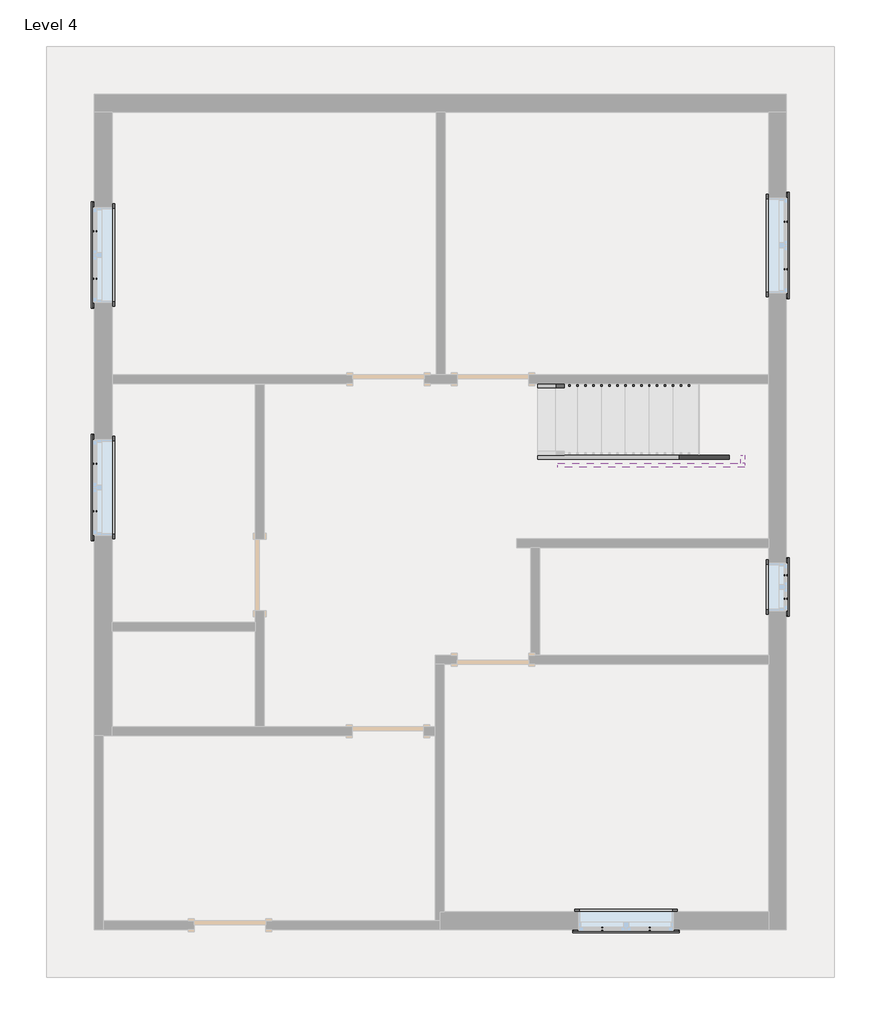
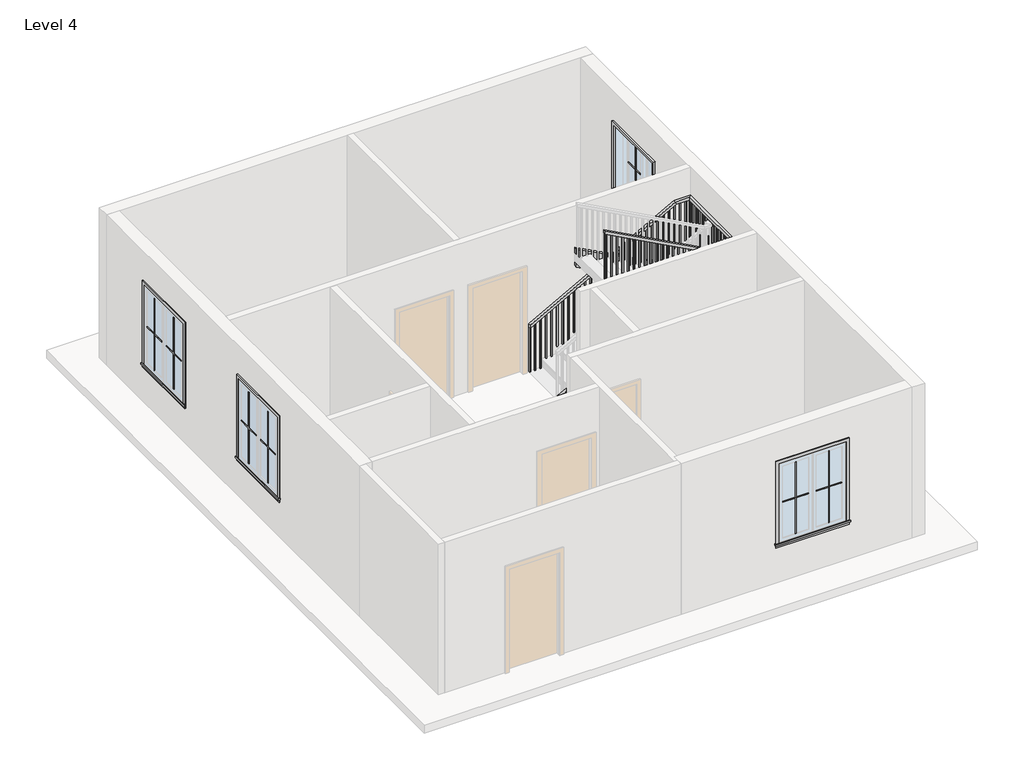
# One storey, part 2 of 2: 20 proxies, 3 members, 1 railing.
"""IFC4 building model written with IfcOpenShell, lengths in millimetres."""

from ifc_helpers import new_model, si_unit, frame, origin, place, context, project, spatial, polyline, outline, extrude, faceted_brep, transform, mapped, element, save
from components import muntin_pattern_2x2_muntin_pattern_2x2_6dad3731, muntin_pattern_2x2_muntin_pattern_2x2_a30a3345, muntin_pattern_2x2_muntin_pattern_2x2_53152e2c, muntin_pattern_2x2_muntin_pattern_2x2_e8f3e573, trim_window_exterior_flat_with_sill_92b9b949, trim_window_exterior_flat_with_sill_a665a915, trim_window_interior_flat_picture_frame_3bb882cf, trim_window_interior_flat_picture_frame_d485c387

model = new_model("IFC4")

# Units and contexts
model_context = context("Model", 3, world=origin())
ifc_project = project(units=[si_unit("LENGTHUNIT", "METRE", prefix="MILLI")], contexts=[model_context])

# Site, building, storey
site = spatial("IfcSite", under=ifc_project)
building = spatial("IfcBuilding", under=site)
storey = spatial("IfcBuildingStorey", under=building, Name="Level 4", Elevation=9144.0)

# Proxies
placement = place(None, origin())
muntin_pattern_2x2_muntin_pattern_2x2_shape = muntin_pattern_2x2_muntin_pattern_2x2_6dad3731(model_context)
element("IfcBuildingElementProxy", 1, Name="Muntin Pattern_2x2 : Muntin Pattern_2x2", ObjectType="Muntin Pattern_2x2 : Muntin Pattern_2x2", at=placement, inside=storey, context=model_context, shape_type="MappedRepresentation", body=[
    mapped(muntin_pattern_2x2_muntin_pattern_2x2_shape, transform((10003.63125, 2232.025, 10128.25), x_axis=(-1.0, 0.0, 0.0), y_axis=(0.0, -1.0, 0.0), z_axis=(0.0, 0.0, 1.0))),
])
element("IfcBuildingElementProxy", 2, Name="Muntin Pattern_2x2 : Muntin Pattern_2x2", ObjectType="Muntin Pattern_2x2 : Muntin Pattern_2x2", at=placement, inside=storey, context=model_context, shape_type="MappedRepresentation", body=[
    mapped(muntin_pattern_2x2_muntin_pattern_2x2_shape, transform((2917.825, 7567.6125, 10128.25), x_axis=(0.0, 1.0, 0.0), y_axis=(-1.0, 0.0, 0.0), z_axis=(0.0, 0.0, 1.0))),
])
element("IfcBuildingElementProxy", 3, Name="Muntin Pattern_2x2 : Muntin Pattern_2x2", ObjectType="Muntin Pattern_2x2 : Muntin Pattern_2x2", at=placement, inside=storey, context=model_context, shape_type="MappedRepresentation", body=[
    mapped(muntin_pattern_2x2_muntin_pattern_2x2_shape, transform((2917.825, 10536.2375, 10128.25), x_axis=(0.0, 1.0, 0.0), y_axis=(-1.0, 0.0, 0.0), z_axis=(0.0, 0.0, 1.0))),
])
element("IfcBuildingElementProxy", 4, Name="Muntin Pattern_2x2 : Muntin Pattern_2x2", ObjectType="Muntin Pattern_2x2 : Muntin Pattern_2x2", at=placement, inside=storey, context=model_context, shape_type="MappedRepresentation", body=[
    mapped(muntin_pattern_2x2_muntin_pattern_2x2_shape, transform((11737.975, 11264.9, 10128.25), x_axis=(0.0, -1.0, 0.0), y_axis=(1.0, 0.0, 0.0), z_axis=(0.0, 0.0, 1.0))),
])
muntin_pattern_2x2_muntin_pattern_2x2_2_shape = muntin_pattern_2x2_muntin_pattern_2x2_a30a3345(model_context)
element("IfcBuildingElementProxy", 5, Name="Muntin Pattern_2x2 : Muntin Pattern_2x2", ObjectType="Muntin Pattern_2x2 : Muntin Pattern_2x2", at=placement, inside=storey, context=model_context, shape_type="MappedRepresentation", body=[
    mapped(muntin_pattern_2x2_muntin_pattern_2x2_2_shape, transform((9397.20625, 2232.025, 10128.25), x_axis=(1.0, 0.0, 0.0), y_axis=(0.0, 1.0, 0.0), z_axis=(0.0, 0.0, 1.0))),
])
element("IfcBuildingElementProxy", 6, Name="Muntin Pattern_2x2 : Muntin Pattern_2x2", ObjectType="Muntin Pattern_2x2 : Muntin Pattern_2x2", at=placement, inside=storey, context=model_context, shape_type="MappedRepresentation", body=[
    mapped(muntin_pattern_2x2_muntin_pattern_2x2_2_shape, transform((2917.825, 8174.0375, 10128.25), x_axis=(0.0, -1.0, 0.0), y_axis=(1.0, 0.0, 0.0), z_axis=(0.0, 0.0, 1.0))),
])
element("IfcBuildingElementProxy", 7, Name="Muntin Pattern_2x2 : Muntin Pattern_2x2", ObjectType="Muntin Pattern_2x2 : Muntin Pattern_2x2", at=placement, inside=storey, context=model_context, shape_type="MappedRepresentation", body=[
    mapped(muntin_pattern_2x2_muntin_pattern_2x2_2_shape, transform((2917.825, 11142.6625, 10128.25), x_axis=(0.0, -1.0, 0.0), y_axis=(1.0, 0.0, 0.0), z_axis=(0.0, 0.0, 1.0))),
])
element("IfcBuildingElementProxy", 8, Name="Muntin Pattern_2x2 : Muntin Pattern_2x2", ObjectType="Muntin Pattern_2x2 : Muntin Pattern_2x2", at=placement, inside=storey, context=model_context, shape_type="MappedRepresentation", body=[
    mapped(muntin_pattern_2x2_muntin_pattern_2x2_2_shape, transform((11737.975, 10658.475, 10128.25), x_axis=(0.0, 1.0, 0.0), y_axis=(-1.0, 0.0, 0.0), z_axis=(0.0, 0.0, 1.0))),
])
muntin_pattern_2x2_muntin_pattern_2x2_3_shape = muntin_pattern_2x2_muntin_pattern_2x2_53152e2c(model_context)
element("IfcBuildingElementProxy", 9, Name="Muntin Pattern_2x2 : Muntin Pattern_2x2", ObjectType="Muntin Pattern_2x2 : Muntin Pattern_2x2", at=placement, inside=storey, context=model_context, shape_type="MappedRepresentation", body=[
    mapped(muntin_pattern_2x2_muntin_pattern_2x2_3_shape, transform((11737.975, 6748.4625, 10128.25), x_axis=(0.0, -1.0, 0.0), y_axis=(1.0, 0.0, 0.0), z_axis=(0.0, 0.0, 1.0))),
])
muntin_pattern_2x2_muntin_pattern_2x2_4_shape = muntin_pattern_2x2_muntin_pattern_2x2_e8f3e573(model_context)
element("IfcBuildingElementProxy", 10, Name="Muntin Pattern_2x2 : Muntin Pattern_2x2", ObjectType="Muntin Pattern_2x2 : Muntin Pattern_2x2", at=placement, inside=storey, context=model_context, shape_type="MappedRepresentation", body=[
    mapped(muntin_pattern_2x2_muntin_pattern_2x2_4_shape, transform((11737.975, 6446.8375, 10128.25), x_axis=(0.0, 1.0, 0.0), y_axis=(-1.0, 0.0, 0.0), z_axis=(0.0, 0.0, 1.0))),
])
trim_window_exterior_flat_with_sill_shape = trim_window_exterior_flat_with_sill_92b9b949(model_context)
element("IfcBuildingElementProxy", 11, Name="Trim-Window-Exterior-Flat : with Sill", ObjectType="Trim-Window-Exterior-Flat : with Sill", at=placement, inside=storey, context=model_context, shape_type="MappedRepresentation", body=[
    mapped(trim_window_exterior_flat_with_sill_shape, transform((9700.41875, 2222.5, 11582.4), x_axis=(1.0, 0.0, 0.0), y_axis=(0.0, 0.0, 1.0), z_axis=(0.0, -1.0, 0.0))),
])
element("IfcBuildingElementProxy", 12, Name="Trim-Window-Exterior-Flat : with Sill", ObjectType="Trim-Window-Exterior-Flat : with Sill", at=placement, inside=storey, context=model_context, shape_type="MappedRepresentation", body=[
    mapped(trim_window_exterior_flat_with_sill_shape, transform((2908.3, 7870.825, 11582.4), x_axis=(0.0, -1.0, 0.0), y_axis=(0.0, 0.0, 1.0), z_axis=(-1.0, 0.0, 0.0))),
])
element("IfcBuildingElementProxy", 13, Name="Trim-Window-Exterior-Flat : with Sill", ObjectType="Trim-Window-Exterior-Flat : with Sill", at=placement, inside=storey, context=model_context, shape_type="MappedRepresentation", body=[
    mapped(trim_window_exterior_flat_with_sill_shape, transform((2908.3, 10839.45, 11582.4), x_axis=(0.0, -1.0, 0.0), y_axis=(0.0, 0.0, 1.0), z_axis=(-1.0, 0.0, 0.0))),
])
element("IfcBuildingElementProxy", 14, Name="Trim-Window-Exterior-Flat : with Sill", ObjectType="Trim-Window-Exterior-Flat : with Sill", at=placement, inside=storey, context=model_context, shape_type="MappedRepresentation", body=[
    mapped(trim_window_exterior_flat_with_sill_shape, transform((11747.5, 10961.6875, 11582.4), x_axis=(0.0, 1.0, 0.0), y_axis=(0.0, 0.0, 1.0), z_axis=(1.0, 0.0, 0.0))),
])
trim_window_exterior_flat_with_sill_2_shape = trim_window_exterior_flat_with_sill_a665a915(model_context)
element("IfcBuildingElementProxy", 15, Name="Trim-Window-Exterior-Flat : with Sill", ObjectType="Trim-Window-Exterior-Flat : with Sill", at=placement, inside=storey, context=model_context, shape_type="MappedRepresentation", body=[
    mapped(trim_window_exterior_flat_with_sill_2_shape, transform((11747.5, 6597.65, 10972.8), x_axis=(0.0, 1.0, 0.0), y_axis=(0.0, 0.0, 1.0), z_axis=(1.0, 0.0, 0.0))),
])
trim_window_interior_flat_picture_frame_shape = trim_window_interior_flat_picture_frame_3bb882cf(model_context)
element("IfcBuildingElementProxy", 16, Name="Trim-Window-Interior-Flat : Picture Frame", ObjectType="Trim-Window-Interior-Flat : Picture Frame", at=placement, inside=storey, context=model_context, shape_type="MappedRepresentation", body=[
    mapped(trim_window_interior_flat_picture_frame_shape, transform((9700.41875, 2451.1, 11582.4), x_axis=(-1.0, 0.0, 0.0), y_axis=(0.0, 0.0, 1.0), z_axis=(0.0, 1.0, 0.0))),
])
element("IfcBuildingElementProxy", 17, Name="Trim-Window-Interior-Flat : Picture Frame", ObjectType="Trim-Window-Interior-Flat : Picture Frame", at=placement, inside=storey, context=model_context, shape_type="MappedRepresentation", body=[
    mapped(trim_window_interior_flat_picture_frame_shape, transform((3136.9, 7870.825, 11582.4), x_axis=(0.0, 1.0, 0.0), y_axis=(0.0, 0.0, 1.0), z_axis=(1.0, 0.0, 0.0))),
])
element("IfcBuildingElementProxy", 18, Name="Trim-Window-Interior-Flat : Picture Frame", ObjectType="Trim-Window-Interior-Flat : Picture Frame", at=placement, inside=storey, context=model_context, shape_type="MappedRepresentation", body=[
    mapped(trim_window_interior_flat_picture_frame_shape, transform((3136.9, 10839.45, 11582.4), x_axis=(0.0, 1.0, 0.0), y_axis=(0.0, 0.0, 1.0), z_axis=(1.0, 0.0, 0.0))),
])
element("IfcBuildingElementProxy", 19, Name="Trim-Window-Interior-Flat : Picture Frame", ObjectType="Trim-Window-Interior-Flat : Picture Frame", at=placement, inside=storey, context=model_context, shape_type="MappedRepresentation", body=[
    mapped(trim_window_interior_flat_picture_frame_shape, transform((11518.9, 10961.6875, 11582.4), x_axis=(0.0, -1.0, 0.0), y_axis=(0.0, 0.0, 1.0), z_axis=(-1.0, 0.0, 0.0))),
])
trim_window_interior_flat_picture_frame_2_shape = trim_window_interior_flat_picture_frame_d485c387(model_context)
element("IfcBuildingElementProxy", 20, Name="Trim-Window-Interior-Flat : Picture Frame", ObjectType="Trim-Window-Interior-Flat : Picture Frame", at=placement, inside=storey, context=model_context, shape_type="MappedRepresentation", body=[
    mapped(trim_window_interior_flat_picture_frame_2_shape, transform((11518.9, 6597.65, 10972.8), x_axis=(0.0, -1.0, 0.0), y_axis=(0.0, 0.0, 1.0), z_axis=(-1.0, 0.0, 0.0))),
])

# Members
element("IfcMember", 21, ObjectType="Stringer - 2\" Width", at=placement, inside=storey, context=model_context, shape_type="SweptSolid", body=[
    extrude(outline(polyline([(9388.4581083, 8572.5), (9144.0, 8572.5), (9144.0, 8761.9689927), (10421.1621978, 11163.3), (10766.3905183, 11163.3), (9388.4581083, 8572.5)])), frame((0.0, 8229.6, 0.0), z_axis=(0.0, 1.0, 0.0), x_axis=(0.0, 0.0, 1.0)), (0.0, 0.0, 1.0), 50.8),
])
element("IfcMember", 22, ObjectType="Stringer - 2\" Width", at=placement, inside=storey, context=model_context, shape_type="SweptSolid", body=[
    extrude(outline(polyline([(11163.3, 8280.4), (11214.1, 8280.4), (11214.1, 8178.8), (11163.3, 8178.8), (11163.3, 8280.4)])), frame((0.0, 0.0, 10519.6105263), z_axis=(0.0, 0.0, 1.0), x_axis=(1.0, 0.0, 0.0)), (0.0, 0.0, 1.0), 304.8),
])
element("IfcMember", 23, ObjectType="Stringer - 2\" Width", at=placement, inside=storey, context=model_context, shape_type="SweptSolid", body=[
    extrude(outline(polyline([(10608.9419568, 11214.1), (10953.380564, 11214.1), (12210.012143, 8826.5), (11865.5735358, 8826.5), (10608.9419568, 11214.1)])), frame((0.0, 8128.0, 0.0), z_axis=(0.0, 1.0, 0.0), x_axis=(0.0, 0.0, 1.0)), (0.0, 0.0, 1.0), 50.8),
])

# Railing
element("IfcRailing", 24, ObjectType="Handrail - Rectangular", at=placement, inside=storey, context=model_context, shape_type="SolidModel", body=[
    faceted_brep([(8572.5, 9194.8, 10218.8210526), (8572.5, 9194.8, 10160.9285199), (8572.5, 9144.0, 10160.9285199), (8572.5, 9144.0, 10218.8210526), (11214.1, 9194.8, 11662.6105263), (11227.076708, 9194.8, 11611.8105263), (11227.076708, 9144.0, 11611.8105263), (11214.1, 9144.0, 11662.6105263), (11518.9, 9194.8, 11662.6105263), (11518.9, 9194.8, 11611.8105263), (11468.1, 9144.0, 11611.8105263), (11468.1, 9144.0, 11662.6105263), (11518.9, 7340.6, 11662.6105263), (11518.9, 7289.8, 11611.8105263), (11468.1, 7289.8, 11611.8105263), (11468.1, 7340.6, 11662.6105263), (11518.9, 7340.6, 11727.4615901), (11518.9, 7289.8, 11676.6615901), (11468.1, 7289.8, 11676.6615901), (11468.1, 7340.6, 11727.4615901), (11518.9, 7213.6, 11727.4615901), (11518.9, 7213.6, 11676.6615901), (11468.1, 7264.4, 11676.6615901), (11468.1, 7264.4, 11727.4615901), (11391.9, 7213.6, 11727.4615901), (11379.1122768, 7213.6, 11676.6615901), (11379.1122768, 7264.4, 11676.6615901), (11391.9, 7264.4, 11727.4615901), (8826.5, 7213.6, 13106.4), (8826.5, 7264.4, 13106.4), (8826.5, 7264.4, 13048.7264198), (8826.5, 7213.6, 13048.7264198)], [[[0, 1, 2, 3]], [[1, 0, 4, 5]], [[2, 1, 5, 6]], [[3, 2, 6, 7]], [[0, 3, 7, 4]], [[5, 4, 8, 9]], [[6, 5, 9, 10]], [[7, 6, 10, 11]], [[4, 7, 11, 8]], [[9, 8, 12, 13]], [[10, 9, 13, 14]], [[11, 10, 14, 15]], [[8, 11, 15, 12]], [[13, 12, 16, 17]], [[14, 13, 17, 18]], [[15, 14, 18, 19]], [[12, 15, 19, 16]], [[17, 16, 20, 21]], [[18, 17, 21, 22]], [[19, 18, 22, 23]], [[16, 19, 23, 20]], [[21, 20, 24, 25]], [[22, 21, 25, 26]], [[23, 22, 26, 27]], [[20, 23, 27, 24]], [[28, 29, 30, 31]], [[25, 24, 28, 31]], [[26, 25, 31, 30]], [[27, 26, 30, 29]], [[24, 27, 29, 28]]]),
    extrude(outline(polyline([(13040.193385, 8842.375), (12031.5789474, 8842.375), (12031.5789474, 8861.425), (13029.9537434, 8861.425), (13040.193385, 8842.375)])), frame((0.0, 7229.475, 0.0), z_axis=(0.0, 1.0, 0.0), x_axis=(0.0, 0.0, 1.0)), (0.0, 0.0, 1.0), 19.05),
    extrude(outline(polyline([(12985.5819629, 8943.975), (12031.5789474, 8943.975), (12031.5789474, 8963.025), (12975.3423212, 8963.025), (12985.5819629, 8943.975)])), frame((0.0, 7229.475, 0.0), z_axis=(0.0, 1.0, 0.0), x_axis=(0.0, 0.0, 1.0)), (0.0, 0.0, 1.0), 19.05),
    extrude(outline(polyline([(12930.9705407, 9045.575), (12031.5789474, 9045.575), (12031.5789474, 9064.625), (12920.730899, 9064.625), (12930.9705407, 9045.575)])), frame((0.0, 7229.475, 0.0), z_axis=(0.0, 1.0, 0.0), x_axis=(0.0, 0.0, 1.0)), (0.0, 0.0, 1.0), 19.05),
    extrude(outline(polyline([(12876.3591185, 9147.175), (11871.1578947, 9147.175), (11871.1578947, 9166.225), (12866.1194769, 9166.225), (12876.3591185, 9147.175)])), frame((0.0, 7229.475, 0.0), z_axis=(0.0, 1.0, 0.0), x_axis=(0.0, 0.0, 1.0)), (0.0, 0.0, 1.0), 19.05),
    extrude(outline(polyline([(12821.7476964, 9248.775), (11871.1578947, 9248.775), (11871.1578947, 9267.825), (12811.5080547, 9267.825), (12821.7476964, 9248.775)])), frame((0.0, 7229.475, 0.0), z_axis=(0.0, 1.0, 0.0), x_axis=(0.0, 0.0, 1.0)), (0.0, 0.0, 1.0), 19.05),
    extrude(outline(polyline([(12767.1362742, 9350.375), (11871.1578947, 9350.375), (11871.1578947, 9369.425), (12756.8966325, 9369.425), (12767.1362742, 9350.375)])), frame((0.0, 7229.475, 0.0), z_axis=(0.0, 1.0, 0.0), x_axis=(0.0, 0.0, 1.0)), (0.0, 0.0, 1.0), 19.05),
    extrude(outline(polyline([(12712.524852, 9451.975), (11710.7368421, 9451.975), (11710.7368421, 9471.025), (12702.2852104, 9471.025), (12712.524852, 9451.975)])), frame((0.0, 7229.475, 0.0), z_axis=(0.0, 1.0, 0.0), x_axis=(0.0, 0.0, 1.0)), (0.0, 0.0, 1.0), 19.05),
    extrude(outline(polyline([(12657.9134298, 9553.575), (11710.7368421, 9553.575), (11710.7368421, 9572.625), (12647.6737882, 9572.625), (12657.9134298, 9553.575)])), frame((0.0, 7229.475, 0.0), z_axis=(0.0, 1.0, 0.0), x_axis=(0.0, 0.0, 1.0)), (0.0, 0.0, 1.0), 19.05),
    extrude(outline(polyline([(12603.3004835, 9655.175), (11710.7368421, 9655.175), (11710.7368421, 9674.225), (12592.8885402, 9674.225), (12603.3004835, 9655.175)])), frame((0.0, 7229.475, 0.0), z_axis=(0.0, 1.0, 0.0), x_axis=(0.0, 0.0, 1.0)), (0.0, 0.0, 1.0), 19.05),
    extrude(outline(polyline([(12548.6905855, 9756.775), (11550.3157895, 9756.775), (11550.3157895, 9775.825), (12538.4509438, 9775.825), (12548.6905855, 9756.775)])), frame((0.0, 7229.475, 0.0), z_axis=(0.0, 1.0, 0.0), x_axis=(0.0, 0.0, 1.0)), (0.0, 0.0, 1.0), 19.05),
    extrude(outline(polyline([(12494.0791633, 9858.375), (11550.3157895, 9858.375), (11550.3157895, 9877.425), (12483.8395217, 9877.425), (12494.0791633, 9858.375)])), frame((0.0, 7229.475, 0.0), z_axis=(0.0, 1.0, 0.0), x_axis=(0.0, 0.0, 1.0)), (0.0, 0.0, 1.0), 19.05),
    extrude(outline(polyline([(12439.4677411, 9959.975), (11550.3157895, 9959.975), (11550.3157895, 9979.025), (12429.2280995, 9979.025), (12439.4677411, 9959.975)])), frame((0.0, 7229.475, 0.0), z_axis=(0.0, 1.0, 0.0), x_axis=(0.0, 0.0, 1.0)), (0.0, 0.0, 1.0), 19.05),
    extrude(outline(polyline([(12384.856319, 10061.575), (11389.8947368, 10061.575), (11389.8947368, 10080.625), (12374.6166773, 10080.625), (12384.856319, 10061.575)])), frame((0.0, 7229.475, 0.0), z_axis=(0.0, 1.0, 0.0), x_axis=(0.0, 0.0, 1.0)), (0.0, 0.0, 1.0), 19.05),
    extrude(outline(polyline([(12330.2448968, 10163.175), (11389.8947368, 10163.175), (11389.8947368, 10182.225), (12320.0052551, 10182.225), (12330.2448968, 10163.175)])), frame((0.0, 7229.475, 0.0), z_axis=(0.0, 1.0, 0.0), x_axis=(0.0, 0.0, 1.0)), (0.0, 0.0, 1.0), 19.05),
    extrude(outline(polyline([(12275.6334746, 10264.775), (11389.8947368, 10264.775), (11389.8947368, 10283.825), (12265.393833, 10283.825), (12275.6334746, 10264.775)])), frame((0.0, 7229.475, 0.0), z_axis=(0.0, 1.0, 0.0), x_axis=(0.0, 0.0, 1.0)), (0.0, 0.0, 1.0), 19.05),
    extrude(outline(polyline([(12221.0220525, 10366.375), (11229.4736842, 10366.375), (11229.4736842, 10385.425), (12210.7824108, 10385.425), (12221.0220525, 10366.375)])), frame((0.0, 7229.475, 0.0), z_axis=(0.0, 1.0, 0.0), x_axis=(0.0, 0.0, 1.0)), (0.0, 0.0, 1.0), 19.05),
    extrude(outline(polyline([(12166.4106303, 10467.975), (11229.4736842, 10467.975), (11229.4736842, 10487.025), (12156.1709886, 10487.025), (12166.4106303, 10467.975)])), frame((0.0, 7229.475, 0.0), z_axis=(0.0, 1.0, 0.0), x_axis=(0.0, 0.0, 1.0)), (0.0, 0.0, 1.0), 19.05),
    extrude(outline(polyline([(12111.7992081, 10569.575), (11229.4736842, 10569.575), (11229.4736842, 10588.625), (12101.5595665, 10588.625), (12111.7992081, 10569.575)])), frame((0.0, 7229.475, 0.0), z_axis=(0.0, 1.0, 0.0), x_axis=(0.0, 0.0, 1.0)), (0.0, 0.0, 1.0), 19.05),
    extrude(outline(polyline([(12057.1877859, 10671.175), (11069.0526316, 10671.175), (11069.0526316, 10690.225), (12046.9481443, 10690.225), (12057.1877859, 10671.175)])), frame((0.0, 7229.475, 0.0), z_axis=(0.0, 1.0, 0.0), x_axis=(0.0, 0.0, 1.0)), (0.0, 0.0, 1.0), 19.05),
    extrude(outline(polyline([(12002.5763638, 10772.775), (11069.0526316, 10772.775), (11069.0526316, 10791.825), (11992.3367221, 10791.825), (12002.5763638, 10772.775)])), frame((0.0, 7229.475, 0.0), z_axis=(0.0, 1.0, 0.0), x_axis=(0.0, 0.0, 1.0)), (0.0, 0.0, 1.0), 19.05),
    extrude(outline(polyline([(11947.9649416, 10874.375), (11069.0526316, 10874.375), (11069.0526316, 10893.425), (11937.7252999, 10893.425), (11947.9649416, 10874.375)])), frame((0.0, 7229.475, 0.0), z_axis=(0.0, 1.0, 0.0), x_axis=(0.0, 0.0, 1.0)), (0.0, 0.0, 1.0), 19.05),
    extrude(outline(polyline([(11893.3535194, 10975.975), (10908.6315789, 10975.975), (10908.6315789, 10995.025), (11883.1138778, 10995.025), (11893.3535194, 10975.975)])), frame((0.0, 7229.475, 0.0), z_axis=(0.0, 1.0, 0.0), x_axis=(0.0, 0.0, 1.0)), (0.0, 0.0, 1.0), 19.05),
    extrude(outline(polyline([(11838.7420972, 11077.575), (10908.6315789, 11077.575), (10908.6315789, 11096.625), (11828.5024556, 11096.625), (11838.7420972, 11077.575)])), frame((0.0, 7229.475, 0.0), z_axis=(0.0, 1.0, 0.0), x_axis=(0.0, 0.0, 1.0)), (0.0, 0.0, 1.0), 19.05),
    extrude(outline(polyline([(11784.1306751, 11179.175), (10908.6315789, 11179.175), (10908.6315789, 11198.225), (11773.8910334, 11198.225), (11784.1306751, 11179.175)])), frame((0.0, 7229.475, 0.0), z_axis=(0.0, 1.0, 0.0), x_axis=(0.0, 0.0, 1.0)), (0.0, 0.0, 1.0), 19.05),
    extrude(outline(polyline([(11729.5192529, 11280.775), (10748.2105263, 11280.775), (10748.2105263, 11299.825), (11719.2796112, 11299.825), (11729.5192529, 11280.775)])), frame((0.0, 7229.475, 0.0), z_axis=(0.0, 1.0, 0.0), x_axis=(0.0, 0.0, 1.0)), (0.0, 0.0, 1.0), 19.05),
    extrude(outline(polyline([(11674.9078307, 11382.375), (10748.2105263, 11382.375), (10748.2105263, 11401.425), (11664.6681891, 11401.425), (11674.9078307, 11382.375)])), frame((0.0, 7229.475, 0.0), z_axis=(0.0, 1.0, 0.0), x_axis=(0.0, 0.0, 1.0)), (0.0, 0.0, 1.0), 19.05),
    extrude(outline(polyline([(11503.025, 7350.125), (11503.025, 7331.075), (11483.975, 7331.075), (11483.975, 7350.125), (11503.025, 7350.125)])), frame((0.0, 0.0, 10748.2105263), z_axis=(0.0, 0.0, 1.0), x_axis=(1.0, 0.0, 0.0)), (0.0, 0.0, 1.0), 863.6),
    extrude(outline(polyline([(11503.025, 7451.725), (11503.025, 7432.675), (11483.975, 7432.675), (11483.975, 7451.725), (11503.025, 7451.725)])), frame((0.0, 0.0, 10748.2105263), z_axis=(0.0, 0.0, 1.0), x_axis=(1.0, 0.0, 0.0)), (0.0, 0.0, 1.0), 863.6),
    extrude(outline(polyline([(11503.025, 7553.325), (11503.025, 7534.275), (11483.975, 7534.275), (11483.975, 7553.325), (11503.025, 7553.325)])), frame((0.0, 0.0, 10748.2105263), z_axis=(0.0, 0.0, 1.0), x_axis=(1.0, 0.0, 0.0)), (0.0, 0.0, 1.0), 863.6),
    extrude(outline(polyline([(11503.025, 7654.925), (11503.025, 7635.875), (11483.975, 7635.875), (11483.975, 7654.925), (11503.025, 7654.925)])), frame((0.0, 0.0, 10748.2105263), z_axis=(0.0, 0.0, 1.0), x_axis=(1.0, 0.0, 0.0)), (0.0, 0.0, 1.0), 863.6),
    extrude(outline(polyline([(11503.025, 7756.525), (11503.025, 7737.475), (11483.975, 7737.475), (11483.975, 7756.525), (11503.025, 7756.525)])), frame((0.0, 0.0, 10748.2105263), z_axis=(0.0, 0.0, 1.0), x_axis=(1.0, 0.0, 0.0)), (0.0, 0.0, 1.0), 863.6),
    extrude(outline(polyline([(11503.025, 7858.125), (11503.025, 7839.075), (11483.975, 7839.075), (11483.975, 7858.125), (11503.025, 7858.125)])), frame((0.0, 0.0, 10748.2105263), z_axis=(0.0, 0.0, 1.0), x_axis=(1.0, 0.0, 0.0)), (0.0, 0.0, 1.0), 863.6),
    extrude(outline(polyline([(11503.025, 7959.725), (11503.025, 7940.675), (11483.975, 7940.675), (11483.975, 7959.725), (11503.025, 7959.725)])), frame((0.0, 0.0, 10748.2105263), z_axis=(0.0, 0.0, 1.0), x_axis=(1.0, 0.0, 0.0)), (0.0, 0.0, 1.0), 863.6),
    extrude(outline(polyline([(11503.025, 8061.325), (11503.025, 8042.275), (11483.975, 8042.275), (11483.975, 8061.325), (11503.025, 8061.325)])), frame((0.0, 0.0, 10748.2105263), z_axis=(0.0, 0.0, 1.0), x_axis=(1.0, 0.0, 0.0)), (0.0, 0.0, 1.0), 863.6),
    extrude(outline(polyline([(11503.025, 8162.925), (11503.025, 8143.875), (11483.975, 8143.875), (11483.975, 8162.925), (11503.025, 8162.925)])), frame((0.0, 0.0, 10748.2105263), z_axis=(0.0, 0.0, 1.0), x_axis=(1.0, 0.0, 0.0)), (0.0, 0.0, 1.0), 863.6),
    extrude(outline(polyline([(11503.025, 8264.525), (11503.025, 8245.475), (11483.975, 8245.475), (11483.975, 8264.525), (11503.025, 8264.525)])), frame((0.0, 0.0, 10748.2105263), z_axis=(0.0, 0.0, 1.0), x_axis=(1.0, 0.0, 0.0)), (0.0, 0.0, 1.0), 863.6),
    extrude(outline(polyline([(11503.025, 8366.125), (11503.025, 8347.075), (11483.975, 8347.075), (11483.975, 8366.125), (11503.025, 8366.125)])), frame((0.0, 0.0, 10748.2105263), z_axis=(0.0, 0.0, 1.0), x_axis=(1.0, 0.0, 0.0)), (0.0, 0.0, 1.0), 863.6),
    extrude(outline(polyline([(11503.025, 8467.725), (11503.025, 8448.675), (11483.975, 8448.675), (11483.975, 8467.725), (11503.025, 8467.725)])), frame((0.0, 0.0, 10748.2105263), z_axis=(0.0, 0.0, 1.0), x_axis=(1.0, 0.0, 0.0)), (0.0, 0.0, 1.0), 863.6),
    extrude(outline(polyline([(11503.025, 8569.325), (11503.025, 8550.275), (11483.975, 8550.275), (11483.975, 8569.325), (11503.025, 8569.325)])), frame((0.0, 0.0, 10748.2105263), z_axis=(0.0, 0.0, 1.0), x_axis=(1.0, 0.0, 0.0)), (0.0, 0.0, 1.0), 863.6),
    extrude(outline(polyline([(11503.025, 8670.925), (11503.025, 8651.875), (11483.975, 8651.875), (11483.975, 8670.925), (11503.025, 8670.925)])), frame((0.0, 0.0, 10748.2105263), z_axis=(0.0, 0.0, 1.0), x_axis=(1.0, 0.0, 0.0)), (0.0, 0.0, 1.0), 863.6),
    extrude(outline(polyline([(11503.025, 8772.525), (11503.025, 8753.475), (11483.975, 8753.475), (11483.975, 8772.525), (11503.025, 8772.525)])), frame((0.0, 0.0, 10748.2105263), z_axis=(0.0, 0.0, 1.0), x_axis=(1.0, 0.0, 0.0)), (0.0, 0.0, 1.0), 863.6),
    extrude(outline(polyline([(11503.025, 8874.125), (11503.025, 8855.075), (11483.975, 8855.075), (11483.975, 8874.125), (11503.025, 8874.125)])), frame((0.0, 0.0, 10748.2105263), z_axis=(0.0, 0.0, 1.0), x_axis=(1.0, 0.0, 0.0)), (0.0, 0.0, 1.0), 863.6),
    extrude(outline(polyline([(11503.025, 8975.725), (11503.025, 8956.675), (11483.975, 8956.675), (11483.975, 8975.725), (11503.025, 8975.725)])), frame((0.0, 0.0, 10748.2105263), z_axis=(0.0, 0.0, 1.0), x_axis=(1.0, 0.0, 0.0)), (0.0, 0.0, 1.0), 863.6),
    extrude(outline(polyline([(11503.025, 9077.325), (11503.025, 9058.275), (11483.975, 9058.275), (11483.975, 9077.325), (11503.025, 9077.325)])), frame((0.0, 0.0, 10748.2105263), z_axis=(0.0, 0.0, 1.0), x_axis=(1.0, 0.0, 0.0)), (0.0, 0.0, 1.0), 863.6),
    extrude(outline(polyline([(11407.775, 9178.925), (11426.825, 9178.925), (11426.825, 9159.875), (11407.775, 9159.875), (11407.775, 9178.925)])), frame((0.0, 0.0, 10748.2105263), z_axis=(0.0, 0.0, 1.0), x_axis=(1.0, 0.0, 0.0)), (0.0, 0.0, 1.0), 863.6),
    extrude(outline(polyline([(11306.175, 9178.925), (11325.225, 9178.925), (11325.225, 9159.875), (11306.175, 9159.875), (11306.175, 9178.925)])), frame((0.0, 0.0, 10748.2105263), z_axis=(0.0, 0.0, 1.0), x_axis=(1.0, 0.0, 0.0)), (0.0, 0.0, 1.0), 863.6),
    extrude(outline(polyline([(11599.512022, 11204.575), (10748.2105263, 11204.575), (10748.2105263, 11223.625), (11609.9239653, 11223.625), (11599.512022, 11204.575)])), frame((0.0, 9159.875, 0.0), z_axis=(0.0, 1.0, 0.0), x_axis=(0.0, 0.0, 1.0)), (0.0, 0.0, 1.0), 19.05),
    extrude(outline(polyline([(11543.9816576, 11102.975), (10587.7894737, 11102.975), (10587.7894737, 11122.025), (11554.3936009, 11122.025), (11543.9816576, 11102.975)])), frame((0.0, 9159.875, 0.0), z_axis=(0.0, 1.0, 0.0), x_axis=(0.0, 0.0, 1.0)), (0.0, 0.0, 1.0), 19.05),
    extrude(outline(polyline([(11488.4512932, 11001.375), (10587.7894737, 11001.375), (10587.7894737, 11020.425), (11498.8632365, 11020.425), (11488.4512932, 11001.375)])), frame((0.0, 9159.875, 0.0), z_axis=(0.0, 1.0, 0.0), x_axis=(0.0, 0.0, 1.0)), (0.0, 0.0, 1.0), 19.05),
    extrude(outline(polyline([(11432.9209288, 10899.775), (10587.7894737, 10899.775), (10587.7894737, 10918.825), (11443.3328722, 10918.825), (11432.9209288, 10899.775)])), frame((0.0, 9159.875, 0.0), z_axis=(0.0, 1.0, 0.0), x_axis=(0.0, 0.0, 1.0)), (0.0, 0.0, 1.0), 19.05),
    extrude(outline(polyline([(11377.3905645, 10798.175), (10427.3684211, 10798.175), (10427.3684211, 10817.225), (11387.8025078, 10817.225), (11377.3905645, 10798.175)])), frame((0.0, 9159.875, 0.0), z_axis=(0.0, 1.0, 0.0), x_axis=(0.0, 0.0, 1.0)), (0.0, 0.0, 1.0), 19.05),
    extrude(outline(polyline([(11321.8602001, 10696.575), (10427.3684211, 10696.575), (10427.3684211, 10715.625), (11332.2721434, 10715.625), (11321.8602001, 10696.575)])), frame((0.0, 9159.875, 0.0), z_axis=(0.0, 1.0, 0.0), x_axis=(0.0, 0.0, 1.0)), (0.0, 0.0, 1.0), 19.05),
    extrude(outline(polyline([(11266.3298357, 10594.975), (10427.3684211, 10594.975), (10427.3684211, 10614.025), (11276.741779, 10614.025), (11266.3298357, 10594.975)])), frame((0.0, 9159.875, 0.0), z_axis=(0.0, 1.0, 0.0), x_axis=(0.0, 0.0, 1.0)), (0.0, 0.0, 1.0), 19.05),
    extrude(outline(polyline([(11210.7994714, 10493.375), (10266.9473684, 10493.375), (10266.9473684, 10512.425), (11221.2114147, 10512.425), (11210.7994714, 10493.375)])), frame((0.0, 9159.875, 0.0), z_axis=(0.0, 1.0, 0.0), x_axis=(0.0, 0.0, 1.0)), (0.0, 0.0, 1.0), 19.05),
    extrude(outline(polyline([(11155.269107, 10391.775), (10266.9473684, 10391.775), (10266.9473684, 10410.825), (11165.6810503, 10410.825), (11155.269107, 10391.775)])), frame((0.0, 9159.875, 0.0), z_axis=(0.0, 1.0, 0.0), x_axis=(0.0, 0.0, 1.0)), (0.0, 0.0, 1.0), 19.05),
    extrude(outline(polyline([(11099.7387426, 10290.175), (10266.9473684, 10290.175), (10266.9473684, 10309.225), (11110.1506859, 10309.225), (11099.7387426, 10290.175)])), frame((0.0, 9159.875, 0.0), z_axis=(0.0, 1.0, 0.0), x_axis=(0.0, 0.0, 1.0)), (0.0, 0.0, 1.0), 19.05),
    extrude(outline(polyline([(11044.2083782, 10188.575), (10106.5263158, 10188.575), (10106.5263158, 10207.625), (11054.6203216, 10207.625), (11044.2083782, 10188.575)])), frame((0.0, 9159.875, 0.0), z_axis=(0.0, 1.0, 0.0), x_axis=(0.0, 0.0, 1.0)), (0.0, 0.0, 1.0), 19.05),
    extrude(outline(polyline([(10988.6780139, 10086.975), (10106.5263158, 10086.975), (10106.5263158, 10106.025), (10999.0899572, 10106.025), (10988.6780139, 10086.975)])), frame((0.0, 9159.875, 0.0), z_axis=(0.0, 1.0, 0.0), x_axis=(0.0, 0.0, 1.0)), (0.0, 0.0, 1.0), 19.05),
    extrude(outline(polyline([(10933.1476495, 9985.375), (10106.5263158, 9985.375), (10106.5263158, 10004.425), (10943.5595928, 10004.425), (10933.1476495, 9985.375)])), frame((0.0, 9159.875, 0.0), z_axis=(0.0, 1.0, 0.0), x_axis=(0.0, 0.0, 1.0)), (0.0, 0.0, 1.0), 19.05),
    extrude(outline(polyline([(10877.6172851, 9883.775), (9946.1052632, 9883.775), (9946.1052632, 9902.825), (10888.0292284, 9902.825), (10877.6172851, 9883.775)])), frame((0.0, 9159.875, 0.0), z_axis=(0.0, 1.0, 0.0), x_axis=(0.0, 0.0, 1.0)), (0.0, 0.0, 1.0), 19.05),
    extrude(outline(polyline([(10822.0869207, 9782.175), (9946.1052632, 9782.175), (9946.1052632, 9801.225), (10832.4988641, 9801.225), (10822.0869207, 9782.175)])), frame((0.0, 9159.875, 0.0), z_axis=(0.0, 1.0, 0.0), x_axis=(0.0, 0.0, 1.0)), (0.0, 0.0, 1.0), 19.05),
    extrude(outline(polyline([(10766.5565564, 9680.575), (9946.1052632, 9680.575), (9946.1052632, 9699.625), (10776.9684997, 9699.625), (10766.5565564, 9680.575)])), frame((0.0, 9159.875, 0.0), z_axis=(0.0, 1.0, 0.0), x_axis=(0.0, 0.0, 1.0)), (0.0, 0.0, 1.0), 19.05),
    extrude(outline(polyline([(10711.026192, 9578.975), (9785.6842105, 9578.975), (9785.6842105, 9598.025), (10721.4381353, 9598.025), (10711.026192, 9578.975)])), frame((0.0, 9159.875, 0.0), z_axis=(0.0, 1.0, 0.0), x_axis=(0.0, 0.0, 1.0)), (0.0, 0.0, 1.0), 19.05),
    extrude(outline(polyline([(10655.4958276, 9477.375), (9785.6842105, 9477.375), (9785.6842105, 9496.425), (10665.9077709, 9496.425), (10655.4958276, 9477.375)])), frame((0.0, 9159.875, 0.0), z_axis=(0.0, 1.0, 0.0), x_axis=(0.0, 0.0, 1.0)), (0.0, 0.0, 1.0), 19.05),
    extrude(outline(polyline([(10599.9654633, 9375.775), (9785.6842105, 9375.775), (9785.6842105, 9394.825), (10610.3774066, 9394.825), (10599.9654633, 9375.775)])), frame((0.0, 9159.875, 0.0), z_axis=(0.0, 1.0, 0.0), x_axis=(0.0, 0.0, 1.0)), (0.0, 0.0, 1.0), 19.05),
    extrude(outline(polyline([(10544.4350989, 9274.175), (9625.2631579, 9274.175), (9625.2631579, 9293.225), (10554.8470422, 9293.225), (10544.4350989, 9274.175)])), frame((0.0, 9159.875, 0.0), z_axis=(0.0, 1.0, 0.0), x_axis=(0.0, 0.0, 1.0)), (0.0, 0.0, 1.0), 19.05),
    extrude(outline(polyline([(10488.9047345, 9172.575), (9625.2631579, 9172.575), (9625.2631579, 9191.625), (10499.3166778, 9191.625), (10488.9047345, 9172.575)])), frame((0.0, 9159.875, 0.0), z_axis=(0.0, 1.0, 0.0), x_axis=(0.0, 0.0, 1.0)), (0.0, 0.0, 1.0), 19.05),
    extrude(outline(polyline([(10433.3743701, 9070.975), (9625.2631579, 9070.975), (9625.2631579, 9090.025), (10443.7863135, 9090.025), (10433.3743701, 9070.975)])), frame((0.0, 9159.875, 0.0), z_axis=(0.0, 1.0, 0.0), x_axis=(0.0, 0.0, 1.0)), (0.0, 0.0, 1.0), 19.05),
    extrude(outline(polyline([(10377.8440058, 8969.375), (9464.8421053, 8969.375), (9464.8421053, 8988.425), (10388.2559491, 8988.425), (10377.8440058, 8969.375)])), frame((0.0, 9159.875, 0.0), z_axis=(0.0, 1.0, 0.0), x_axis=(0.0, 0.0, 1.0)), (0.0, 0.0, 1.0), 19.05),
    extrude(outline(polyline([(10322.3136414, 8867.775), (9464.8421053, 8867.775), (9464.8421053, 8886.825), (10332.7255847, 8886.825), (10322.3136414, 8867.775)])), frame((0.0, 9159.875, 0.0), z_axis=(0.0, 1.0, 0.0), x_axis=(0.0, 0.0, 1.0)), (0.0, 0.0, 1.0), 19.05),
    extrude(outline(polyline([(10266.783277, 8766.175), (9304.4210526, 8766.175), (9304.4210526, 8785.225), (10277.1952203, 8785.225), (10266.783277, 8766.175)])), frame((0.0, 9159.875, 0.0), z_axis=(0.0, 1.0, 0.0), x_axis=(0.0, 0.0, 1.0)), (0.0, 0.0, 1.0), 19.05),
    extrude(outline(polyline([(10211.2529126, 8664.575), (9304.4210526, 8664.575), (9304.4210526, 8683.625), (10221.664856, 8683.625), (10211.2529126, 8664.575)])), frame((0.0, 9159.875, 0.0), z_axis=(0.0, 1.0, 0.0), x_axis=(0.0, 0.0, 1.0)), (0.0, 0.0, 1.0), 19.05),
    extrude(outline(polyline([(11503.025, 7248.525), (11503.025, 7229.475), (11483.975, 7229.475), (11483.975, 7248.525), (11503.025, 7248.525)])), frame((0.0, 0.0, 10748.2105263), z_axis=(0.0, 0.0, 1.0), x_axis=(1.0, 0.0, 0.0)), (0.0, 0.0, 1.0), 928.4510638),
    extrude(outline(polyline([(11483.975, 9178.925), (11503.025, 9178.925), (11503.025, 9159.875), (11483.975, 9159.875), (11483.975, 9178.925)])), frame((0.0, 0.0, 10748.2105263), z_axis=(0.0, 0.0, 1.0), x_axis=(1.0, 0.0, 0.0)), (0.0, 0.0, 1.0), 863.6),
    extrude(outline(polyline([(13048.7264198, 8826.5), (12031.5789474, 8826.5), (12031.5789474, 8845.55), (13038.4867781, 8845.55), (13048.7264198, 8826.5)])), frame((0.0, 7229.475, 0.0), z_axis=(0.0, 1.0, 0.0), x_axis=(0.0, 0.0, 1.0)), (0.0, 0.0, 1.0), 19.05),
    extrude(outline(polyline([(10160.9285199, 8572.5), (9304.4210526, 8572.5), (9304.4210526, 8591.55), (10171.3404633, 8591.55), (10160.9285199, 8572.5)])), frame((0.0, 9159.875, 0.0), z_axis=(0.0, 1.0, 0.0), x_axis=(0.0, 0.0, 1.0)), (0.0, 0.0, 1.0), 19.05),
])

save(model, "model.ifc")

# Revit data of these elements
# Type "Muntin Pattern_2x2 : Muntin Pattern_2x2"
#   Width [instance default] = 4' - 0"
#   Thickness = 0' - 0 1/2"
#   Height [instance default] = 4' - 0"
#   Distance = 0' - 0 3/4"
#   Interior Material [instance default] = none
#   Exterior Material [instance default] = none
#   Default Elevation = 0
# Type "Trim-Window-Exterior-Flat : with Sill"
#   Trim Width = 0' - 2 1/4"
#   Trim Thickness_Picture Frame = 0' - 1 1/4"
#   Trim Thickness_with Sill = 0' - 0 3/4"
#   Sill Thickness = 0' - 1 1/4"
#   Opening Width [instance default] = 2' - 0"
#   Opening Height [instance default] = 3' - 0"
#   Default Elevation = 4' - 0"
#   Sill = yes
#   Picture Frame = no
#   Trim Material [instance default] = none
# Type "Trim-Window-Interior-Flat : Picture Frame"
#   Trim Thickness_Picture Frame = 0' - 1 1/4"
#   Trim Width = 0' - 2 1/4"
#   Trim Thickness_with Sill = 0' - 0 3/4"
#   Sill Thickness = 0' - 1 1/4"
#   Opening Width [instance default] = 2' - 0"
#   Opening Height [instance default] = 3' - 0"
#   Default Elevation = 4' - 0"
#   Sill = no
#   Picture Frame = yes
#   Trim Material [instance default] = none
# Type "Handrail - Rectangular"
#   Assembly Code = "C2010400"
#   built-in parameter 1008612 = 0.0416667 (stored number, unit not read)
#   built-in parameter 1008611 = 0.0416667 (stored number, unit not read)
#   built-in parameter 1008609 = 0.333333 (stored number, unit not read)
#   built-in parameter 1008604 = 0.166667 (stored number, unit not read)
#   built-in parameter 1008603 = 0.166667 (stored number, unit not read)
#   Railing Height = 3' - 0"
#   built-in parameter 1008630 = 2
#   built-in parameter 1008610 = 2
#   built-in parameter 1008618 = Baluster - Square : 3/4"
# Elements 1, 2, 3, 4, 5, 6, 7, 8 (IfcBuildingElementProxy, "Muntin Pattern_2x2 : Muntin Pattern_2x2")
#   Width = 1' - 6 5/8"
#   Height = 4' - 6 1/2"
#   Interior Material = Wood - Stained
#   Exterior Material = Clad - White
#   Phase Created = New Construction
#   Materials on its faces: "Clad - White", "Wood - Stained"
# Elements 9, 10 (IfcBuildingElementProxy, "Muntin Pattern_2x2 : Muntin Pattern_2x2")
#   Width = 0' - 6 5/8"
#   Height = 2' - 6 1/2"
#   Interior Material = Wood - Stained
#   Exterior Material = Clad - White
#   Phase Created = New Construction
#   Materials on its faces: "Clad - White", "Wood - Stained"
# Elements 11, 12, 13, 14 (IfcBuildingElementProxy, "Trim-Window-Exterior-Flat : with Sill")
#   Opening Width = 4' - 0"
#   Opening Height = 5' - 0"
#   Trim Material = Clad - White
#   Phase Created = New Construction
#   Materials on its faces: "Clad - White"
# Element 15 (IfcBuildingElementProxy, "Trim-Window-Exterior-Flat : with Sill")
#   Opening Width = 2' - 0"
#   Opening Height = 3' - 0"
#   Trim Material = Clad - White
#   Phase Created = New Construction
#   Materials on its faces: "Clad - White"
# Elements 16, 17, 18, 19 (IfcBuildingElementProxy, "Trim-Window-Interior-Flat : Picture Frame")
#   Opening Width = 4' - 0"
#   Opening Height = 5' - 0"
#   Trim Material = Wood - Stained
#   Phase Created = New Construction
#   Materials on its faces: "Wood - Stained"
# Element 20 (IfcBuildingElementProxy, "Trim-Window-Interior-Flat : Picture Frame")
#   Opening Width = 2' - 0"
#   Opening Height = 3' - 0"
#   Trim Material = Wood - Stained
#   Phase Created = New Construction
#   Materials on its faces: "Wood - Stained"
# Elements 21, 22, 23 (IfcMember, "Stringer - 2\" Width")
#   Phase Created = New Construction
# Element 24 (IfcRailing, "Handrail - Rectangular")
#   Phase Created = New Construction
# Materials
#   "Clad - White": class "Wood", colour RGB 242 242 238, transparency 0, Cost = 0
#   "Wood - Stained": class "Wood", colour RGB 224 178 126, transparency 0, Cost = 0
